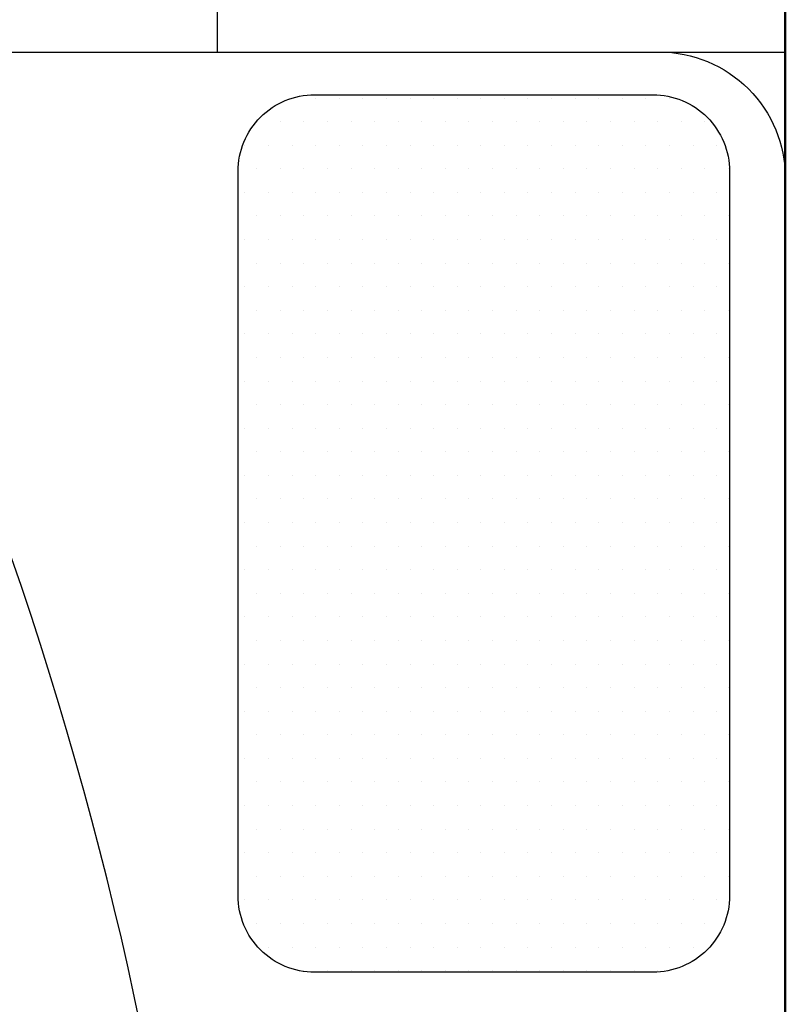
# Model space of a CAD drawing. Units: inches. Extents: x 3064 to 19385, y 846 to 15425.
# Tile 15 of 108: x 3758 to 3782, y 1063 to 1094. Entities that reach past the tile are written whole.
import ezdxf

# ---------------------------------------------------------------- set-up
doc = ezdxf.new("R2010")
doc.units = ezdxf.units.IN
doc.layers.add('A-FLOR-FIXT', color=9, linetype='Continuous', lineweight=18)
doc.layers.add('A-WALL', color=7, linetype='Continuous', lineweight=50)
doc.layers.add('BLOCK', color=6, linetype='Continuous')

# ---------------------------------------------------------------- blocks, each defined once
blk = doc.blocks.new('*X7')
at = {"color": 0}
for p, q in [((266.4375, 457.03125), (266.4375, 457.03125)), ((266.8125, 457.03125), (266.8125, 457.03125)), ((267.1875, 457.03125), (267.1875, 457.03125)), ((267.5625, 457.03125), (267.5625, 457.03125)), ((267.9375, 457.03125), (267.9375, 457.03125)), ((268.3125, 457.03125), (268.3125, 457.03125)), ((268.6875, 457.03125), (268.6875, 457.03125)), ((269.0625, 457.03125), (269.0625, 457.03125)), ((269.4375, 457.03125), (269.4375, 457.03125)), ((269.8125, 457.03125), (269.8125, 457.03125)), ((270.1875, 457.03125), (270.1875, 457.03125)), ((270.5625, 457.03125), (270.5625, 457.03125)), ((270.9375, 457.03125), (270.9375, 457.03125)), ((271.3125, 457.03125), (271.3125, 457.03125)), ((271.6875, 457.03125), (271.6875, 457.03125)), ((272.0625, 457.03125), (272.0625, 457.03125)), ((266.25, 456.9375), (266.25, 456.9375)), ((266.625, 456.9375), (266.625, 456.9375)), ((267, 456.9375), (267, 456.9375)), ((267.375, 456.9375), (267.375, 456.9375)), ((267.75, 456.9375), (267.75, 456.9375)), ((268.125, 456.9375), (268.125, 456.9375)), ((268.5, 456.9375), (268.5, 456.9375)), ((268.875, 456.9375), (268.875, 456.9375)), ((269.25, 456.9375), (269.25, 456.9375)), ((269.625, 456.9375), (269.625, 456.9375)), ((270, 456.9375), (270, 456.9375)), ((270.375, 456.9375), (270.375, 456.9375)), ((270.75, 456.9375), (270.75, 456.9375)), ((271.125, 456.9375), (271.125, 456.9375)), ((271.5, 456.9375), (271.5, 456.9375)), ((271.875, 456.9375), (271.875, 456.9375)), ((272.25, 456.9375), (272.25, 456.9375)), ((266.0625, 456.84375), (266.0625, 456.84375)), ((266.4375, 456.84375), (266.4375, 456.84375)), ((266.8125, 456.84375), (266.8125, 456.84375)), ((267.1875, 456.84375), (267.1875, 456.84375)), ((267.5625, 456.84375), (267.5625, 456.84375)), ((267.9375, 456.84375), (267.9375, 456.84375)), ((268.3125, 456.84375), (268.3125, 456.84375)), ((268.6875, 456.84375), (268.6875, 456.84375)), ((269.0625, 456.84375), (269.0625, 456.84375)), ((269.4375, 456.84375), (269.4375, 456.84375)), ((269.8125, 456.84375), (269.8125, 456.84375)), ((270.1875, 456.84375), (270.1875, 456.84375)), ((270.5625, 456.84375), (270.5625, 456.84375)), ((270.9375, 456.84375), (270.9375, 456.84375)), ((271.3125, 456.84375), (271.3125, 456.84375)), ((271.6875, 456.84375), (271.6875, 456.84375)), ((272.0625, 456.84375), (272.0625, 456.84375)), ((272.4375, 456.84375), (272.4375, 456.84375)), ((266.25, 456.75), (266.25, 456.75)), ((266.625, 456.75), (266.625, 456.75)), ((267, 456.75), (267, 456.75)), ((267.375, 456.75), (267.375, 456.75)), ((267.75, 456.75), (267.75, 456.75)), ((268.125, 456.75), (268.125, 456.75)), ((268.5, 456.75), (268.5, 456.75)), ((268.875, 456.75), (268.875, 456.75)), ((269.25, 456.75), (269.25, 456.75)), ((269.625, 456.75), (269.625, 456.75)), ((270, 456.75), (270, 456.75)), ((270.375, 456.75), (270.375, 456.75)), ((270.75, 456.75), (270.75, 456.75)), ((271.125, 456.75), (271.125, 456.75)), ((271.5, 456.75), (271.5, 456.75)), ((271.875, 456.75), (271.875, 456.75)), ((272.25, 456.75), (272.25, 456.75)), ((272.625, 456.75), (272.625, 456.75)), ((266.0625, 456.65625), (266.0625, 456.65625)), ((266.4375, 456.65625), (266.4375, 456.65625)), ((266.8125, 456.65625), (266.8125, 456.65625)), ((267.1875, 456.65625), (267.1875, 456.65625)), ((267.5625, 456.65625), (267.5625, 456.65625)), ((267.9375, 456.65625), (267.9375, 456.65625)), ((268.3125, 456.65625), (268.3125, 456.65625)), ((268.6875, 456.65625), (268.6875, 456.65625)), ((269.0625, 456.65625), (269.0625, 456.65625)), ((269.4375, 456.65625), (269.4375, 456.65625)), ((269.8125, 456.65625), (269.8125, 456.65625)), ((270.1875, 456.65625), (270.1875, 456.65625)), ((270.5625, 456.65625), (270.5625, 456.65625)), ((270.9375, 456.65625), (270.9375, 456.65625)), ((271.3125, 456.65625), (271.3125, 456.65625)), ((271.6875, 456.65625), (271.6875, 456.65625)), ((272.0625, 456.65625), (272.0625, 456.65625)), ((272.4375, 456.65625), (272.4375, 456.65625)), ((265.875, 456.5625), (265.875, 456.5625)), ((266.25, 456.5625), (266.25, 456.5625)), ((266.625, 456.5625), (266.625, 456.5625)), ((267, 456.5625), (267, 456.5625)), ((267.375, 456.5625), (267.375, 456.5625)), ((267.75, 456.5625), (267.75, 456.5625)), ((268.125, 456.5625), (268.125, 456.5625)), ((268.5, 456.5625), (268.5, 456.5625)), ((268.875, 456.5625), (268.875, 456.5625)), ((269.25, 456.5625), (269.25, 456.5625)), ((269.625, 456.5625), (269.625, 456.5625)), ((270, 456.5625), (270, 456.5625)), ((270.375, 456.5625), (270.375, 456.5625)), ((270.75, 456.5625), (270.75, 456.5625)), ((271.125, 456.5625), (271.125, 456.5625)), ((271.5, 456.5625), (271.5, 456.5625)), ((271.875, 456.5625), (271.875, 456.5625)), ((272.25, 456.5625), (272.25, 456.5625)), ((272.625, 456.5625), (272.625, 456.5625)), ((266.0625, 456.46875), (266.0625, 456.46875)), ((266.4375, 456.46875), (266.4375, 456.46875)), ((266.8125, 456.46875), (266.8125, 456.46875)), ((267.1875, 456.46875), (267.1875, 456.46875)), ((267.5625, 456.46875), (267.5625, 456.46875)), ((267.9375, 456.46875), (267.9375, 456.46875)), ((268.3125, 456.46875), (268.3125, 456.46875)), ((268.6875, 456.46875), (268.6875, 456.46875)), ((269.0625, 456.46875), (269.0625, 456.46875)), ((269.4375, 456.46875), (269.4375, 456.46875)), ((269.8125, 456.46875), (269.8125, 456.46875)), ((270.1875, 456.46875), (270.1875, 456.46875)), ((270.5625, 456.46875), (270.5625, 456.46875)), ((270.9375, 456.46875), (270.9375, 456.46875)), ((271.3125, 456.46875), (271.3125, 456.46875)), ((271.6875, 456.46875), (271.6875, 456.46875)), ((272.0625, 456.46875), (272.0625, 456.46875)), ((272.4375, 456.46875), (272.4375, 456.46875)), ((272.8125, 456.46875), (272.8125, 456.46875)), ((265.875, 456.375), (265.875, 456.375)), ((266.25, 456.375), (266.25, 456.375)), ((266.625, 456.375), (266.625, 456.375)), ((267, 456.375), (267, 456.375)), ((267.375, 456.375), (267.375, 456.375)), ((267.75, 456.375), (267.75, 456.375)), ((268.125, 456.375), (268.125, 456.375)), ((268.5, 456.375), (268.5, 456.375)), ((268.875, 456.375), (268.875, 456.375)), ((269.25, 456.375), (269.25, 456.375)), ((269.625, 456.375), (269.625, 456.375)), ((270, 456.375), (270, 456.375)), ((270.375, 456.375), (270.375, 456.375)), ((270.75, 456.375), (270.75, 456.375)), ((271.125, 456.375), (271.125, 456.375)), ((271.5, 456.375), (271.5, 456.375)), ((271.875, 456.375), (271.875, 456.375)), ((272.25, 456.375), (272.25, 456.375)), ((272.625, 456.375), (272.625, 456.375)), ((266.0625, 456.28125), (266.0625, 456.28125)), ((266.4375, 456.28125), (266.4375, 456.28125)), ((266.8125, 456.28125), (266.8125, 456.28125)), ((267.1875, 456.28125), (267.1875, 456.28125)), ((267.5625, 456.28125), (267.5625, 456.28125)), ((267.9375, 456.28125), (267.9375, 456.28125)), ((268.3125, 456.28125), (268.3125, 456.28125)), ((268.6875, 456.28125), (268.6875, 456.28125)), ((269.0625, 456.28125), (269.0625, 456.28125)), ((269.4375, 456.28125), (269.4375, 456.28125)), ((269.8125, 456.28125), (269.8125, 456.28125)), ((270.1875, 456.28125), (270.1875, 456.28125)), ((270.5625, 456.28125), (270.5625, 456.28125)), ((270.9375, 456.28125), (270.9375, 456.28125)), ((271.3125, 456.28125), (271.3125, 456.28125)), ((271.6875, 456.28125), (271.6875, 456.28125)), ((272.0625, 456.28125), (272.0625, 456.28125)), ((272.4375, 456.28125), (272.4375, 456.28125)), ((272.8125, 456.28125), (272.8125, 456.28125)), ((265.875, 456.1875), (265.875, 456.1875)), ((266.25, 456.1875), (266.25, 456.1875)), ((266.625, 456.1875), (266.625, 456.1875)), ((267, 456.1875), (267, 456.1875)), ((267.375, 456.1875), (267.375, 456.1875)), ((267.75, 456.1875), (267.75, 456.1875)), ((268.125, 456.1875), (268.125, 456.1875)), ((268.5, 456.1875), (268.5, 456.1875)), ((268.875, 456.1875), (268.875, 456.1875)), ((269.25, 456.1875), (269.25, 456.1875)), ((269.625, 456.1875), (269.625, 456.1875)), ((270, 456.1875), (270, 456.1875)), ((270.375, 456.1875), (270.375, 456.1875)), ((270.75, 456.1875), (270.75, 456.1875)), ((271.125, 456.1875), (271.125, 456.1875)), ((271.5, 456.1875), (271.5, 456.1875)), ((271.875, 456.1875), (271.875, 456.1875)), ((272.25, 456.1875), (272.25, 456.1875)), ((272.625, 456.1875), (272.625, 456.1875)), ((266.0625, 456.09375), (266.0625, 456.09375)), ((266.4375, 456.09375), (266.4375, 456.09375)), ((266.8125, 456.09375), (266.8125, 456.09375)), ((267.1875, 456.09375), (267.1875, 456.09375)), ((267.5625, 456.09375), (267.5625, 456.09375)), ((267.9375, 456.09375), (267.9375, 456.09375)), ((268.3125, 456.09375), (268.3125, 456.09375)), ((268.6875, 456.09375), (268.6875, 456.09375)), ((269.0625, 456.09375), (269.0625, 456.09375)), ((269.4375, 456.09375), (269.4375, 456.09375)), ((269.8125, 456.09375), (269.8125, 456.09375)), ((270.1875, 456.09375), (270.1875, 456.09375)), ((270.5625, 456.09375), (270.5625, 456.09375)), ((270.9375, 456.09375), (270.9375, 456.09375)), ((271.3125, 456.09375), (271.3125, 456.09375)), ((271.6875, 456.09375), (271.6875, 456.09375)), ((272.0625, 456.09375), (272.0625, 456.09375)), ((272.4375, 456.09375), (272.4375, 456.09375)), ((272.8125, 456.09375), (272.8125, 456.09375)), ((265.875, 456), (265.875, 456)), ((266.25, 456), (266.25, 456)), ((266.625, 456), (266.625, 456)), ((267, 456), (267, 456)), ((267.375, 456), (267.375, 456)), ((267.75, 456), (267.75, 456)), ((268.125, 456), (268.125, 456)), ((268.5, 456), (268.5, 456)), ((268.875, 456), (268.875, 456)), ((269.25, 456), (269.25, 456)), ((269.625, 456), (269.625, 456)), ((270, 456), (270, 456)), ((270.375, 456), (270.375, 456)), ((270.75, 456), (270.75, 456)), ((271.125, 456), (271.125, 456)), ((271.5, 456), (271.5, 456)), ((271.875, 456), (271.875, 456)), ((272.25, 456), (272.25, 456)), ((272.625, 456), (272.625, 456)), ((266.0625, 455.90625), (266.0625, 455.90625)), ((266.4375, 455.90625), (266.4375, 455.90625)), ((266.8125, 455.90625), (266.8125, 455.90625)), ((267.1875, 455.90625), (267.1875, 455.90625)), ((267.5625, 455.90625), (267.5625, 455.90625)), ((267.9375, 455.90625), (267.9375, 455.90625)), ((268.3125, 455.90625), (268.3125, 455.90625)), ((268.6875, 455.90625), (268.6875, 455.90625)), ((269.0625, 455.90625), (269.0625, 455.90625)), ((269.4375, 455.90625), (269.4375, 455.90625)), ((269.8125, 455.90625), (269.8125, 455.90625)), ((270.1875, 455.90625), (270.1875, 455.90625)), ((270.5625, 455.90625), (270.5625, 455.90625)), ((270.9375, 455.90625), (270.9375, 455.90625)), ((271.3125, 455.90625), (271.3125, 455.90625)), ((271.6875, 455.90625), (271.6875, 455.90625)), ((272.0625, 455.90625), (272.0625, 455.90625)), ((272.4375, 455.90625), (272.4375, 455.90625)), ((272.8125, 455.90625), (272.8125, 455.90625)), ((265.875, 455.8125), (265.875, 455.8125)), ((266.25, 455.8125), (266.25, 455.8125)), ((266.625, 455.8125), (266.625, 455.8125)), ((267, 455.8125), (267, 455.8125)), ((267.375, 455.8125), (267.375, 455.8125)), ((267.75, 455.8125), (267.75, 455.8125)), ((268.125, 455.8125), (268.125, 455.8125)), ((268.5, 455.8125), (268.5, 455.8125)), ((268.875, 455.8125), (268.875, 455.8125)), ((269.25, 455.8125), (269.25, 455.8125)), ((269.625, 455.8125), (269.625, 455.8125)), ((270, 455.8125), (270, 455.8125)), ((270.375, 455.8125), (270.375, 455.8125)), ((270.75, 455.8125), (270.75, 455.8125)), ((271.125, 455.8125), (271.125, 455.8125)), ((271.5, 455.8125), (271.5, 455.8125)), ((271.875, 455.8125), (271.875, 455.8125)), ((272.25, 455.8125), (272.25, 455.8125)), ((272.625, 455.8125), (272.625, 455.8125)), ((266.0625, 455.71875), (266.0625, 455.71875)), ((266.4375, 455.71875), (266.4375, 455.71875)), ((266.8125, 455.71875), (266.8125, 455.71875)), ((267.1875, 455.71875), (267.1875, 455.71875)), ((267.5625, 455.71875), (267.5625, 455.71875)), ((267.9375, 455.71875), (267.9375, 455.71875)), ((268.3125, 455.71875), (268.3125, 455.71875)), ((268.6875, 455.71875), (268.6875, 455.71875)), ((269.0625, 455.71875), (269.0625, 455.71875)), ((269.4375, 455.71875), (269.4375, 455.71875)), ((269.8125, 455.71875), (269.8125, 455.71875)), ((270.1875, 455.71875), (270.1875, 455.71875)), ((270.5625, 455.71875), (270.5625, 455.71875)), ((270.9375, 455.71875), (270.9375, 455.71875)), ((271.3125, 455.71875), (271.3125, 455.71875)), ((271.6875, 455.71875), (271.6875, 455.71875)), ((272.0625, 455.71875), (272.0625, 455.71875)), ((272.4375, 455.71875), (272.4375, 455.71875)), ((272.8125, 455.71875), (272.8125, 455.71875)), ((265.875, 455.625), (265.875, 455.625)), ((266.25, 455.625), (266.25, 455.625)), ((266.625, 455.625), (266.625, 455.625)), ((267, 455.625), (267, 455.625)), ((267.375, 455.625), (267.375, 455.625)), ((267.75, 455.625), (267.75, 455.625)), ((268.125, 455.625), (268.125, 455.625)), ((268.5, 455.625), (268.5, 455.625)), ((268.875, 455.625), (268.875, 455.625)), ((269.25, 455.625), (269.25, 455.625)), ((269.625, 455.625), (269.625, 455.625)), ((270, 455.625), (270, 455.625)), ((270.375, 455.625), (270.375, 455.625)), ((270.75, 455.625), (270.75, 455.625)), ((271.125, 455.625), (271.125, 455.625)), ((271.5, 455.625), (271.5, 455.625)), ((271.875, 455.625), (271.875, 455.625)), ((272.25, 455.625), (272.25, 455.625)), ((272.625, 455.625), (272.625, 455.625)), ((266.0625, 455.53125), (266.0625, 455.53125)), ((266.4375, 455.53125), (266.4375, 455.53125)), ((266.8125, 455.53125), (266.8125, 455.53125)), ((267.1875, 455.53125), (267.1875, 455.53125)), ((267.5625, 455.53125), (267.5625, 455.53125)), ((267.9375, 455.53125), (267.9375, 455.53125)), ((268.3125, 455.53125), (268.3125, 455.53125)), ((268.6875, 455.53125), (268.6875, 455.53125)), ((269.0625, 455.53125), (269.0625, 455.53125)), ((269.4375, 455.53125), (269.4375, 455.53125)), ((269.8125, 455.53125), (269.8125, 455.53125)), ((270.1875, 455.53125), (270.1875, 455.53125)), ((270.5625, 455.53125), (270.5625, 455.53125)), ((270.9375, 455.53125), (270.9375, 455.53125)), ((271.3125, 455.53125), (271.3125, 455.53125)), ((271.6875, 455.53125), (271.6875, 455.53125)), ((272.0625, 455.53125), (272.0625, 455.53125)), ((272.4375, 455.53125), (272.4375, 455.53125)), ((272.8125, 455.53125), (272.8125, 455.53125)), ((265.875, 455.4375), (265.875, 455.4375)), ((266.25, 455.4375), (266.25, 455.4375)), ((266.625, 455.4375), (266.625, 455.4375)), ((267, 455.4375), (267, 455.4375)), ((267.375, 455.4375), (267.375, 455.4375)), ((267.75, 455.4375), (267.75, 455.4375)), ((268.125, 455.4375), (268.125, 455.4375)), ((268.5, 455.4375), (268.5, 455.4375)), ((268.875, 455.4375), (268.875, 455.4375)), ((269.25, 455.4375), (269.25, 455.4375)), ((269.625, 455.4375), (269.625, 455.4375)), ((270, 455.4375), (270, 455.4375)), ((270.375, 455.4375), (270.375, 455.4375)), ((270.75, 455.4375), (270.75, 455.4375)), ((271.125, 455.4375), (271.125, 455.4375)), ((271.5, 455.4375), (271.5, 455.4375)), ((271.875, 455.4375), (271.875, 455.4375)), ((272.25, 455.4375), (272.25, 455.4375)), ((272.625, 455.4375), (272.625, 455.4375)), ((266.0625, 455.34375), (266.0625, 455.34375)), ((266.4375, 455.34375), (266.4375, 455.34375)), ((266.8125, 455.34375), (266.8125, 455.34375)), ((267.1875, 455.34375), (267.1875, 455.34375)), ((267.5625, 455.34375), (267.5625, 455.34375)), ((267.9375, 455.34375), (267.9375, 455.34375)), ((268.3125, 455.34375), (268.3125, 455.34375)), ((268.6875, 455.34375), (268.6875, 455.34375)), ((269.0625, 455.34375), (269.0625, 455.34375)), ((269.4375, 455.34375), (269.4375, 455.34375)), ((269.8125, 455.34375), (269.8125, 455.34375)), ((270.1875, 455.34375), (270.1875, 455.34375)), ((270.5625, 455.34375), (270.5625, 455.34375)), ((270.9375, 455.34375), (270.9375, 455.34375)), ((271.3125, 455.34375), (271.3125, 455.34375)), ((271.6875, 455.34375), (271.6875, 455.34375)), ((272.0625, 455.34375), (272.0625, 455.34375)), ((272.4375, 455.34375), (272.4375, 455.34375)), ((272.8125, 455.34375), (272.8125, 455.34375)), ((265.875, 455.25), (265.875, 455.25)), ((266.25, 455.25), (266.25, 455.25)), ((266.625, 455.25), (266.625, 455.25)), ((267, 455.25), (267, 455.25)), ((267.375, 455.25), (267.375, 455.25)), ((267.75, 455.25), (267.75, 455.25)), ((268.125, 455.25), (268.125, 455.25)), ((268.5, 455.25), (268.5, 455.25)), ((268.875, 455.25), (268.875, 455.25)), ((269.25, 455.25), (269.25, 455.25)), ((269.625, 455.25), (269.625, 455.25)), ((270, 455.25), (270, 455.25)), ((270.375, 455.25), (270.375, 455.25)), ((270.75, 455.25), (270.75, 455.25)), ((271.125, 455.25), (271.125, 455.25)), ((271.5, 455.25), (271.5, 455.25)), ((271.875, 455.25), (271.875, 455.25)), ((272.25, 455.25), (272.25, 455.25)), ((272.625, 455.25), (272.625, 455.25)), ((266.0625, 455.15625), (266.0625, 455.15625)), ((266.4375, 455.15625), (266.4375, 455.15625)), ((266.8125, 455.15625), (266.8125, 455.15625)), ((267.1875, 455.15625), (267.1875, 455.15625)), ((267.5625, 455.15625), (267.5625, 455.15625)), ((267.9375, 455.15625), (267.9375, 455.15625)), ((268.3125, 455.15625), (268.3125, 455.15625)), ((268.6875, 455.15625), (268.6875, 455.15625)), ((269.0625, 455.15625), (269.0625, 455.15625)), ((269.4375, 455.15625), (269.4375, 455.15625)), ((269.8125, 455.15625), (269.8125, 455.15625)), ((270.1875, 455.15625), (270.1875, 455.15625)), ((270.5625, 455.15625), (270.5625, 455.15625)), ((270.9375, 455.15625), (270.9375, 455.15625)), ((271.3125, 455.15625), (271.3125, 455.15625)), ((271.6875, 455.15625), (271.6875, 455.15625)), ((272.0625, 455.15625), (272.0625, 455.15625)), ((272.4375, 455.15625), (272.4375, 455.15625)), ((272.8125, 455.15625), (272.8125, 455.15625)), ((265.875, 455.0625), (265.875, 455.0625)), ((266.25, 455.0625), (266.25, 455.0625)), ((266.625, 455.0625), (266.625, 455.0625)), ((267, 455.0625), (267, 455.0625)), ((267.375, 455.0625), (267.375, 455.0625)), ((267.75, 455.0625), (267.75, 455.0625)), ((268.125, 455.0625), (268.125, 455.0625)), ((268.5, 455.0625), (268.5, 455.0625)), ((268.875, 455.0625), (268.875, 455.0625)), ((269.25, 455.0625), (269.25, 455.0625)), ((269.625, 455.0625), (269.625, 455.0625)), ((270, 455.0625), (270, 455.0625)), ((270.375, 455.0625), (270.375, 455.0625)), ((270.75, 455.0625), (270.75, 455.0625)), ((271.125, 455.0625), (271.125, 455.0625)), ((271.5, 455.0625), (271.5, 455.0625)), ((271.875, 455.0625), (271.875, 455.0625)), ((272.25, 455.0625), (272.25, 455.0625)), ((272.625, 455.0625), (272.625, 455.0625)), ((266.0625, 454.96875), (266.0625, 454.96875)), ((266.4375, 454.96875), (266.4375, 454.96875)), ((266.8125, 454.96875), (266.8125, 454.96875)), ((267.1875, 454.96875), (267.1875, 454.96875)), ((267.5625, 454.96875), (267.5625, 454.96875)), ((267.9375, 454.96875), (267.9375, 454.96875)), ((268.3125, 454.96875), (268.3125, 454.96875)), ((268.6875, 454.96875), (268.6875, 454.96875)), ((269.0625, 454.96875), (269.0625, 454.96875)), ((269.4375, 454.96875), (269.4375, 454.96875)), ((269.8125, 454.96875), (269.8125, 454.96875)), ((270.1875, 454.96875), (270.1875, 454.96875)), ((270.5625, 454.96875), (270.5625, 454.96875)), ((270.9375, 454.96875), (270.9375, 454.96875)), ((271.3125, 454.96875), (271.3125, 454.96875)), ((271.6875, 454.96875), (271.6875, 454.96875)), ((272.0625, 454.96875), (272.0625, 454.96875)), ((272.4375, 454.96875), (272.4375, 454.96875)), ((272.8125, 454.96875), (272.8125, 454.96875)), ((265.875, 454.875), (265.875, 454.875)), ((266.25, 454.875), (266.25, 454.875)), ((266.625, 454.875), (266.625, 454.875)), ((267, 454.875), (267, 454.875)), ((267.375, 454.875), (267.375, 454.875)), ((267.75, 454.875), (267.75, 454.875)), ((268.125, 454.875), (268.125, 454.875)), ((268.5, 454.875), (268.5, 454.875)), ((268.875, 454.875), (268.875, 454.875)), ((269.25, 454.875), (269.25, 454.875)), ((269.625, 454.875), (269.625, 454.875)), ((270, 454.875), (270, 454.875)), ((270.375, 454.875), (270.375, 454.875)), ((270.75, 454.875), (270.75, 454.875)), ((271.125, 454.875), (271.125, 454.875)), ((271.5, 454.875), (271.5, 454.875)), ((271.875, 454.875), (271.875, 454.875)), ((272.25, 454.875), (272.25, 454.875)), ((272.625, 454.875), (272.625, 454.875)), ((266.0625, 454.78125), (266.0625, 454.78125)), ((266.4375, 454.78125), (266.4375, 454.78125)), ((266.8125, 454.78125), (266.8125, 454.78125)), ((267.1875, 454.78125), (267.1875, 454.78125)), ((267.5625, 454.78125), (267.5625, 454.78125)), ((267.9375, 454.78125), (267.9375, 454.78125)), ((268.3125, 454.78125), (268.3125, 454.78125)), ((268.6875, 454.78125), (268.6875, 454.78125)), ((269.0625, 454.78125), (269.0625, 454.78125)), ((269.4375, 454.78125), (269.4375, 454.78125)), ((269.8125, 454.78125), (269.8125, 454.78125)), ((270.1875, 454.78125), (270.1875, 454.78125)), ((270.5625, 454.78125), (270.5625, 454.78125)), ((270.9375, 454.78125), (270.9375, 454.78125)), ((271.3125, 454.78125), (271.3125, 454.78125)), ((271.6875, 454.78125), (271.6875, 454.78125)), ((272.0625, 454.78125), (272.0625, 454.78125)), ((272.4375, 454.78125), (272.4375, 454.78125)), ((272.8125, 454.78125), (272.8125, 454.78125)), ((265.875, 454.6875), (265.875, 454.6875)), ((266.25, 454.6875), (266.25, 454.6875)), ((266.625, 454.6875), (266.625, 454.6875)), ((267, 454.6875), (267, 454.6875)), ((267.375, 454.6875), (267.375, 454.6875)), ((267.75, 454.6875), (267.75, 454.6875)), ((268.125, 454.6875), (268.125, 454.6875)), ((268.5, 454.6875), (268.5, 454.6875)), ((268.875, 454.6875), (268.875, 454.6875)), ((269.25, 454.6875), (269.25, 454.6875)), ((269.625, 454.6875), (269.625, 454.6875)), ((270, 454.6875), (270, 454.6875)), ((270.375, 454.6875), (270.375, 454.6875)), ((270.75, 454.6875), (270.75, 454.6875)), ((271.125, 454.6875), (271.125, 454.6875)), ((271.5, 454.6875), (271.5, 454.6875)), ((271.875, 454.6875), (271.875, 454.6875)), ((272.25, 454.6875), (272.25, 454.6875)), ((272.625, 454.6875), (272.625, 454.6875)), ((266.0625, 454.59375), (266.0625, 454.59375)), ((266.4375, 454.59375), (266.4375, 454.59375)), ((266.8125, 454.59375), (266.8125, 454.59375)), ((267.1875, 454.59375), (267.1875, 454.59375)), ((267.5625, 454.59375), (267.5625, 454.59375)), ((267.9375, 454.59375), (267.9375, 454.59375)), ((268.3125, 454.59375), (268.3125, 454.59375)), ((268.6875, 454.59375), (268.6875, 454.59375)), ((269.0625, 454.59375), (269.0625, 454.59375)), ((269.4375, 454.59375), (269.4375, 454.59375)), ((269.8125, 454.59375), (269.8125, 454.59375)), ((270.1875, 454.59375), (270.1875, 454.59375)), ((270.5625, 454.59375), (270.5625, 454.59375)), ((270.9375, 454.59375), (270.9375, 454.59375)), ((271.3125, 454.59375), (271.3125, 454.59375)), ((271.6875, 454.59375), (271.6875, 454.59375)), ((272.0625, 454.59375), (272.0625, 454.59375)), ((272.4375, 454.59375), (272.4375, 454.59375)), ((272.8125, 454.59375), (272.8125, 454.59375)), ((265.875, 454.5), (265.875, 454.5)), ((266.25, 454.5), (266.25, 454.5)), ((266.625, 454.5), (266.625, 454.5)), ((267, 454.5), (267, 454.5)), ((267.375, 454.5), (267.375, 454.5)), ((267.75, 454.5), (267.75, 454.5)), ((268.125, 454.5), (268.125, 454.5)), ((268.5, 454.5), (268.5, 454.5)), ((268.875, 454.5), (268.875, 454.5)), ((269.25, 454.5), (269.25, 454.5)), ((269.625, 454.5), (269.625, 454.5)), ((270, 454.5), (270, 454.5)), ((270.375, 454.5), (270.375, 454.5)), ((270.75, 454.5), (270.75, 454.5)), ((271.125, 454.5), (271.125, 454.5)), ((271.5, 454.5), (271.5, 454.5)), ((271.875, 454.5), (271.875, 454.5)), ((272.25, 454.5), (272.25, 454.5)), ((272.625, 454.5), (272.625, 454.5)), ((266.0625, 454.40625), (266.0625, 454.40625)), ((266.4375, 454.40625), (266.4375, 454.40625)), ((266.8125, 454.40625), (266.8125, 454.40625)), ((267.1875, 454.40625), (267.1875, 454.40625)), ((267.5625, 454.40625), (267.5625, 454.40625)), ((267.9375, 454.40625), (267.9375, 454.40625)), ((268.3125, 454.40625), (268.3125, 454.40625)), ((268.6875, 454.40625), (268.6875, 454.40625)), ((269.0625, 454.40625), (269.0625, 454.40625)), ((269.4375, 454.40625), (269.4375, 454.40625)), ((269.8125, 454.40625), (269.8125, 454.40625)), ((270.1875, 454.40625), (270.1875, 454.40625)), ((270.5625, 454.40625), (270.5625, 454.40625)), ((270.9375, 454.40625), (270.9375, 454.40625)), ((271.3125, 454.40625), (271.3125, 454.40625)), ((271.6875, 454.40625), (271.6875, 454.40625)), ((272.0625, 454.40625), (272.0625, 454.40625)), ((272.4375, 454.40625), (272.4375, 454.40625)), ((272.8125, 454.40625), (272.8125, 454.40625)), ((265.875, 454.3125), (265.875, 454.3125)), ((266.25, 454.3125), (266.25, 454.3125)), ((266.625, 454.3125), (266.625, 454.3125)), ((267, 454.3125), (267, 454.3125)), ((267.375, 454.3125), (267.375, 454.3125)), ((267.75, 454.3125), (267.75, 454.3125)), ((268.125, 454.3125), (268.125, 454.3125)), ((268.5, 454.3125), (268.5, 454.3125)), ((268.875, 454.3125), (268.875, 454.3125)), ((269.25, 454.3125), (269.25, 454.3125)), ((269.625, 454.3125), (269.625, 454.3125)), ((270, 454.3125), (270, 454.3125)), ((270.375, 454.3125), (270.375, 454.3125)), ((270.75, 454.3125), (270.75, 454.3125)), ((271.125, 454.3125), (271.125, 454.3125)), ((271.5, 454.3125), (271.5, 454.3125)), ((271.875, 454.3125), (271.875, 454.3125)), ((272.25, 454.3125), (272.25, 454.3125)), ((272.625, 454.3125), (272.625, 454.3125)), ((266.0625, 454.21875), (266.0625, 454.21875)), ((266.4375, 454.21875), (266.4375, 454.21875)), ((266.8125, 454.21875), (266.8125, 454.21875)), ((267.1875, 454.21875), (267.1875, 454.21875)), ((267.5625, 454.21875), (267.5625, 454.21875)), ((267.9375, 454.21875), (267.9375, 454.21875)), ((268.3125, 454.21875), (268.3125, 454.21875)), ((268.6875, 454.21875), (268.6875, 454.21875)), ((269.0625, 454.21875), (269.0625, 454.21875)), ((269.4375, 454.21875), (269.4375, 454.21875)), ((269.8125, 454.21875), (269.8125, 454.21875)), ((270.1875, 454.21875), (270.1875, 454.21875)), ((270.5625, 454.21875), (270.5625, 454.21875)), ((270.9375, 454.21875), (270.9375, 454.21875)), ((271.3125, 454.21875), (271.3125, 454.21875)), ((271.6875, 454.21875), (271.6875, 454.21875)), ((272.0625, 454.21875), (272.0625, 454.21875)), ((272.4375, 454.21875), (272.4375, 454.21875)), ((272.8125, 454.21875), (272.8125, 454.21875)), ((265.875, 454.125), (265.875, 454.125)), ((266.25, 454.125), (266.25, 454.125)), ((266.625, 454.125), (266.625, 454.125)), ((267, 454.125), (267, 454.125)), ((267.375, 454.125), (267.375, 454.125)), ((267.75, 454.125), (267.75, 454.125)), ((268.125, 454.125), (268.125, 454.125)), ((268.5, 454.125), (268.5, 454.125)), ((268.875, 454.125), (268.875, 454.125)), ((269.25, 454.125), (269.25, 454.125)), ((269.625, 454.125), (269.625, 454.125)), ((270, 454.125), (270, 454.125)), ((270.375, 454.125), (270.375, 454.125)), ((270.75, 454.125), (270.75, 454.125)), ((271.125, 454.125), (271.125, 454.125)), ((271.5, 454.125), (271.5, 454.125)), ((271.875, 454.125), (271.875, 454.125)), ((272.25, 454.125), (272.25, 454.125)), ((272.625, 454.125), (272.625, 454.125)), ((266.0625, 454.03125), (266.0625, 454.03125)), ((266.4375, 454.03125), (266.4375, 454.03125)), ((266.8125, 454.03125), (266.8125, 454.03125)), ((267.1875, 454.03125), (267.1875, 454.03125)), ((267.5625, 454.03125), (267.5625, 454.03125)), ((267.9375, 454.03125), (267.9375, 454.03125)), ((268.3125, 454.03125), (268.3125, 454.03125)), ((268.6875, 454.03125), (268.6875, 454.03125)), ((269.0625, 454.03125), (269.0625, 454.03125)), ((269.4375, 454.03125), (269.4375, 454.03125)), ((269.8125, 454.03125), (269.8125, 454.03125)), ((270.1875, 454.03125), (270.1875, 454.03125)), ((270.5625, 454.03125), (270.5625, 454.03125)), ((270.9375, 454.03125), (270.9375, 454.03125)), ((271.3125, 454.03125), (271.3125, 454.03125)), ((271.6875, 454.03125), (271.6875, 454.03125)), ((272.0625, 454.03125), (272.0625, 454.03125)), ((272.4375, 454.03125), (272.4375, 454.03125)), ((272.8125, 454.03125), (272.8125, 454.03125)), ((265.875, 453.9375), (265.875, 453.9375)), ((266.25, 453.9375), (266.25, 453.9375)), ((266.625, 453.9375), (266.625, 453.9375)), ((267, 453.9375), (267, 453.9375)), ((267.375, 453.9375), (267.375, 453.9375)), ((267.75, 453.9375), (267.75, 453.9375)), ((268.125, 453.9375), (268.125, 453.9375)), ((268.5, 453.9375), (268.5, 453.9375)), ((268.875, 453.9375), (268.875, 453.9375)), ((269.25, 453.9375), (269.25, 453.9375)), ((269.625, 453.9375), (269.625, 453.9375)), ((270, 453.9375), (270, 453.9375)), ((270.375, 453.9375), (270.375, 453.9375)), ((270.75, 453.9375), (270.75, 453.9375)), ((271.125, 453.9375), (271.125, 453.9375)), ((271.5, 453.9375), (271.5, 453.9375)), ((271.875, 453.9375), (271.875, 453.9375)), ((272.25, 453.9375), (272.25, 453.9375)), ((272.625, 453.9375), (272.625, 453.9375)), ((266.0625, 453.84375), (266.0625, 453.84375)), ((266.4375, 453.84375), (266.4375, 453.84375)), ((266.8125, 453.84375), (266.8125, 453.84375)), ((267.1875, 453.84375), (267.1875, 453.84375)), ((267.5625, 453.84375), (267.5625, 453.84375)), ((267.9375, 453.84375), (267.9375, 453.84375)), ((268.3125, 453.84375), (268.3125, 453.84375)), ((268.6875, 453.84375), (268.6875, 453.84375)), ((269.0625, 453.84375), (269.0625, 453.84375)), ((269.4375, 453.84375), (269.4375, 453.84375)), ((269.8125, 453.84375), (269.8125, 453.84375)), ((270.1875, 453.84375), (270.1875, 453.84375)), ((270.5625, 453.84375), (270.5625, 453.84375)), ((270.9375, 453.84375), (270.9375, 453.84375)), ((271.3125, 453.84375), (271.3125, 453.84375)), ((271.6875, 453.84375), (271.6875, 453.84375)), ((272.0625, 453.84375), (272.0625, 453.84375)), ((272.4375, 453.84375), (272.4375, 453.84375)), ((272.8125, 453.84375), (272.8125, 453.84375)), ((265.875, 453.75), (265.875, 453.75)), ((266.25, 453.75), (266.25, 453.75)), ((266.625, 453.75), (266.625, 453.75)), ((267, 453.75), (267, 453.75)), ((267.375, 453.75), (267.375, 453.75)), ((267.75, 453.75), (267.75, 453.75)), ((268.125, 453.75), (268.125, 453.75)), ((268.5, 453.75), (268.5, 453.75)), ((268.875, 453.75), (268.875, 453.75)), ((269.25, 453.75), (269.25, 453.75)), ((269.625, 453.75), (269.625, 453.75)), ((270, 453.75), (270, 453.75)), ((270.375, 453.75), (270.375, 453.75)), ((270.75, 453.75), (270.75, 453.75)), ((271.125, 453.75), (271.125, 453.75)), ((271.5, 453.75), (271.5, 453.75)), ((271.875, 453.75), (271.875, 453.75)), ((272.25, 453.75), (272.25, 453.75)), ((272.625, 453.75), (272.625, 453.75)), ((266.0625, 453.65625), (266.0625, 453.65625)), ((266.4375, 453.65625), (266.4375, 453.65625)), ((266.8125, 453.65625), (266.8125, 453.65625)), ((267.1875, 453.65625), (267.1875, 453.65625)), ((267.5625, 453.65625), (267.5625, 453.65625)), ((267.9375, 453.65625), (267.9375, 453.65625)), ((268.3125, 453.65625), (268.3125, 453.65625)), ((268.6875, 453.65625), (268.6875, 453.65625)), ((269.0625, 453.65625), (269.0625, 453.65625)), ((269.4375, 453.65625), (269.4375, 453.65625)), ((269.8125, 453.65625), (269.8125, 453.65625)), ((270.1875, 453.65625), (270.1875, 453.65625)), ((270.5625, 453.65625), (270.5625, 453.65625)), ((270.9375, 453.65625), (270.9375, 453.65625)), ((271.3125, 453.65625), (271.3125, 453.65625)), ((271.6875, 453.65625), (271.6875, 453.65625)), ((272.0625, 453.65625), (272.0625, 453.65625)), ((272.4375, 453.65625), (272.4375, 453.65625)), ((272.8125, 453.65625), (272.8125, 453.65625)), ((266.25, 453.5625), (266.25, 453.5625)), ((266.625, 453.5625), (266.625, 453.5625)), ((267, 453.5625), (267, 453.5625)), ((267.375, 453.5625), (267.375, 453.5625)), ((267.75, 453.5625), (267.75, 453.5625)), ((268.125, 453.5625), (268.125, 453.5625)), ((268.5, 453.5625), (268.5, 453.5625)), ((268.875, 453.5625), (268.875, 453.5625)), ((269.25, 453.5625), (269.25, 453.5625)), ((269.625, 453.5625), (269.625, 453.5625)), ((270, 453.5625), (270, 453.5625)), ((270.375, 453.5625), (270.375, 453.5625)), ((270.75, 453.5625), (270.75, 453.5625)), ((271.125, 453.5625), (271.125, 453.5625)), ((271.5, 453.5625), (271.5, 453.5625)), ((271.875, 453.5625), (271.875, 453.5625)), ((272.25, 453.5625), (272.25, 453.5625)), ((272.625, 453.5625), (272.625, 453.5625)), ((266.0625, 453.46875), (266.0625, 453.46875)), ((266.4375, 453.46875), (266.4375, 453.46875)), ((266.8125, 453.46875), (266.8125, 453.46875)), ((267.1875, 453.46875), (267.1875, 453.46875)), ((267.5625, 453.46875), (267.5625, 453.46875)), ((267.9375, 453.46875), (267.9375, 453.46875)), ((268.3125, 453.46875), (268.3125, 453.46875)), ((268.6875, 453.46875), (268.6875, 453.46875)), ((269.0625, 453.46875), (269.0625, 453.46875)), ((269.4375, 453.46875), (269.4375, 453.46875)), ((269.8125, 453.46875), (269.8125, 453.46875)), ((270.1875, 453.46875), (270.1875, 453.46875)), ((270.5625, 453.46875), (270.5625, 453.46875)), ((270.9375, 453.46875), (270.9375, 453.46875)), ((271.3125, 453.46875), (271.3125, 453.46875)), ((271.6875, 453.46875), (271.6875, 453.46875)), ((272.0625, 453.46875), (272.0625, 453.46875)), ((272.4375, 453.46875), (272.4375, 453.46875)), ((266.25, 453.375), (266.25, 453.375)), ((266.625, 453.375), (266.625, 453.375)), ((267, 453.375), (267, 453.375)), ((267.375, 453.375), (267.375, 453.375)), ((267.75, 453.375), (267.75, 453.375)), ((268.125, 453.375), (268.125, 453.375)), ((268.5, 453.375), (268.5, 453.375)), ((268.875, 453.375), (268.875, 453.375)), ((269.25, 453.375), (269.25, 453.375)), ((269.625, 453.375), (269.625, 453.375)), ((270, 453.375), (270, 453.375)), ((270.375, 453.375), (270.375, 453.375)), ((270.75, 453.375), (270.75, 453.375)), ((271.125, 453.375), (271.125, 453.375)), ((271.5, 453.375), (271.5, 453.375)), ((271.875, 453.375), (271.875, 453.375)), ((272.25, 453.375), (272.25, 453.375)), ((272.625, 453.375), (272.625, 453.375)), ((266.0625, 453.28125), (266.0625, 453.28125)), ((266.4375, 453.28125), (266.4375, 453.28125)), ((266.8125, 453.28125), (266.8125, 453.28125)), ((267.1875, 453.28125), (267.1875, 453.28125)), ((267.5625, 453.28125), (267.5625, 453.28125)), ((267.9375, 453.28125), (267.9375, 453.28125)), ((268.3125, 453.28125), (268.3125, 453.28125)), ((268.6875, 453.28125), (268.6875, 453.28125)), ((269.0625, 453.28125), (269.0625, 453.28125)), ((269.4375, 453.28125), (269.4375, 453.28125)), ((269.8125, 453.28125), (269.8125, 453.28125)), ((270.1875, 453.28125), (270.1875, 453.28125)), ((270.5625, 453.28125), (270.5625, 453.28125)), ((270.9375, 453.28125), (270.9375, 453.28125)), ((271.3125, 453.28125), (271.3125, 453.28125)), ((271.6875, 453.28125), (271.6875, 453.28125)), ((272.0625, 453.28125), (272.0625, 453.28125)), ((272.4375, 453.28125), (272.4375, 453.28125)), ((266.25, 453.1875), (266.25, 453.1875)), ((266.625, 453.1875), (266.625, 453.1875)), ((267, 453.1875), (267, 453.1875)), ((267.375, 453.1875), (267.375, 453.1875)), ((267.75, 453.1875), (267.75, 453.1875)), ((268.125, 453.1875), (268.125, 453.1875)), ((268.5, 453.1875), (268.5, 453.1875)), ((268.875, 453.1875), (268.875, 453.1875)), ((269.25, 453.1875), (269.25, 453.1875)), ((269.625, 453.1875), (269.625, 453.1875)), ((270, 453.1875), (270, 453.1875)), ((270.375, 453.1875), (270.375, 453.1875)), ((270.75, 453.1875), (270.75, 453.1875)), ((271.125, 453.1875), (271.125, 453.1875)), ((271.5, 453.1875), (271.5, 453.1875)), ((271.875, 453.1875), (271.875, 453.1875)), ((272.25, 453.1875), (272.25, 453.1875))]:
    blk.add_line(p, q, dxfattribs=at)
blk = doc.blocks.new('A$C52E67D0D')
at = {"layer": 'BLOCK'}
blk.add_lwpolyline([(501, 1348.63), (501, 1799.63), (0, 1799.63), (0, 1348.63)], close=True, dxfattribs=at)
for points in [[(1901, 0), (601, 0, -0.414214), (501, 100), (501, 1700, -0.414214), (601, 1800), (1901, 1800, -0.414214), (2001, 1700), (2001, 100, -0.414214)], [(1171.77, 1365.08), (595.83, 1365.08, -0.414214), (534.98, 1425.93), (534.98, 1694.83, -0.414214), (595.83, 1755.67), (1171.77, 1755.67, -0.414214), (1232.61, 1694.83), (1232.61, 1425.93, -0.414214)]]:
    blk.add_lwpolyline(points, format="xyb", close=True, dxfattribs=at)
for centre, radius, start, end in [((1888.63, -1664.54), 3015.26, 87.86419, 117.40011), ((3101.01, -1685.8), 3227.66, 109.92605, 135.39771)]:
    blk.add_arc(centre, radius, start, end, dxfattribs=at)
at = {"layer": 'BLOCK', "xscale": 100, "yscale": 100, "zscale": 100}
blk.add_blockref('*X7', (-26049.96, -43948.24), dxfattribs=at)

msp = doc.modelspace()

# ---------------------------------------------------------------- linework, layer by layer
at = {"layer": 'A-WALL'}
msp.add_line((3782.359, 1144.34), (3782.359, 982.34), dxfattribs=at)

# ---------------------------------------------------------------- block references
at = {"layer": 'A-FLOR-FIXT', "xscale": 0.039370099999992, "yscale": 0.039370099999992, "zscale": 0.039370099999992, "rotation": 270}
msp.add_blockref('A$C52E67D0D', (3711.493, 1112.592), dxfattribs=at)

doc.saveas('drawing.dxf')
